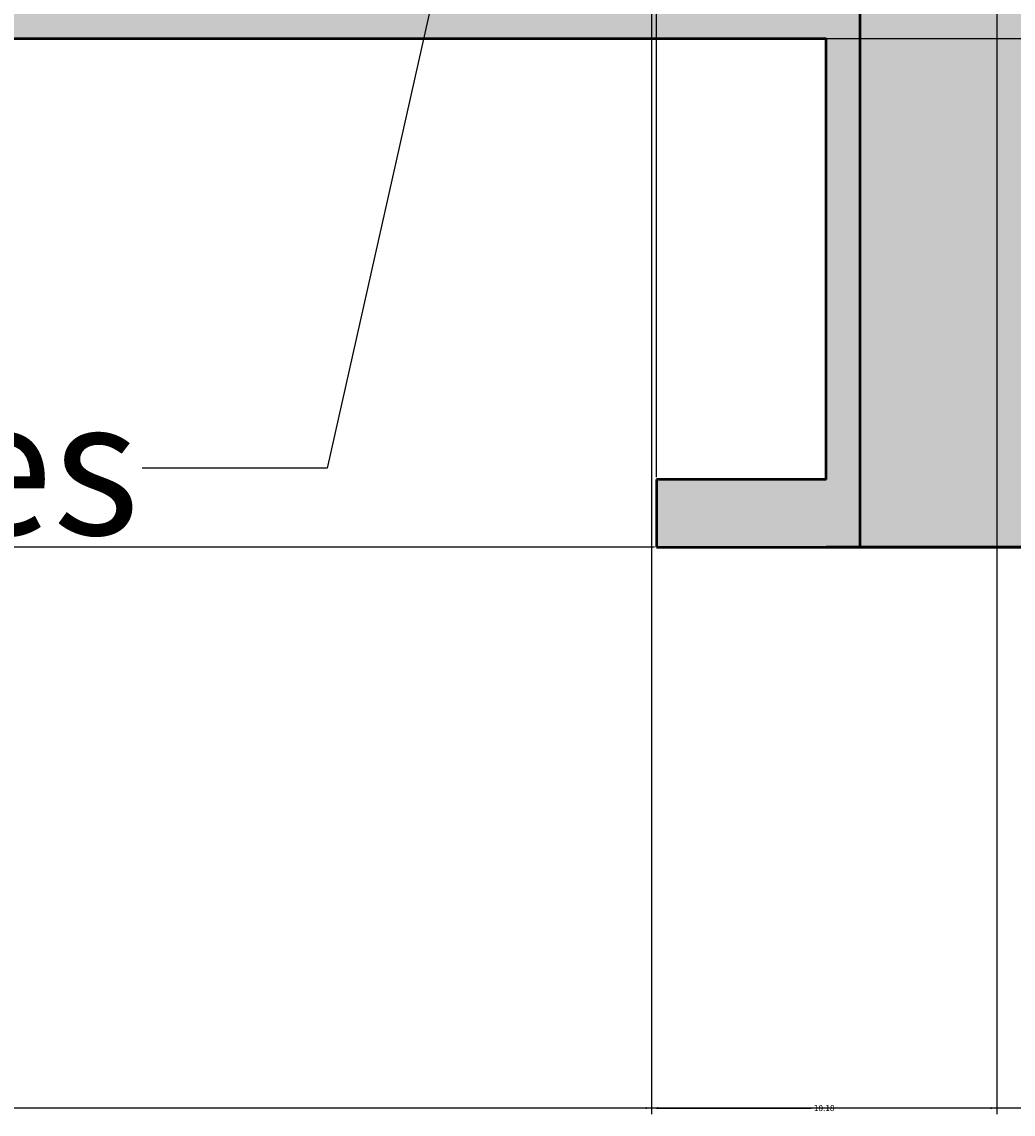
# Model space of a CAD drawing. Units: inches. Extents: x -12 to 334, y -10 to 186.
# Tile 47 of 77: x 198 to 227, y 14 to 46. Entities that reach past the tile are written whole.
import ezdxf
from ezdxf import colors
from ezdxf.entities.mleader import LeaderData, LeaderLine
from ezdxf.math import Vec2, Vec3

# ---------------------------------------------------------------- set-up
doc = ezdxf.new("R2010")
doc.units = ezdxf.units.IN
doc.header["$MEASUREMENT"] = 0
for name, color, linetype, lineweight in [('M-ANNO-TEXT', 3, 'Continuous', 25), ('M-DIMS', 2, 'Continuous', 18), ('M-EQPM', 7, 'Continuous', 50), ('M-EQPM-PATT', 8, 'Continuous', 18)]:
    doc.layers.add(name, color=color, linetype=linetype, lineweight=lineweight)
doc.styles.get("Standard").update_dxf_attribs({"font": 'arial.ttf'})
doc.dimstyles.get("Standard").update_dxf_attribs({"dimtxt": 0.18, "dimasz": 0.18, "dimexe": 0.18, "dimexo": 0.0625, "dimgap": 0.09, "dimtad": 0, "dimtih": 1, "dimtoh": 1, "dimdec": 4, "dimzin": 0, "dimdsep": 46, "dimtxsty": 'Standard', "dimcen": 0.09, "dimadec": 0, "dimazin": 0, "dimtfac": 1, "dimtdec": 4, "dimtofl": 0, "dimtmove": 0, "dimatfit": 3, "dimfxl": 1, "dimtolj": 1, "dimtzin": 0, "dimarcsym": 0})

# ---------------------------------------------------------------- blocks, each defined once
blk = doc.blocks.new('*D1')
at = {"layer": 'Defpoints', "color": 0, "transparency": 16777216}
for p in [(281.426, 91.899), (3.376, 80.692), (281.426, 14.304)]:
    blk.add_point(p, dxfattribs=at)
at = {"layer": 'M-DIMS', "color": 0, "lineweight": -2, "transparency": 16777216}
for p, q in [((281.426, 91.836), (281.426, 14.124)), ((3.376, 80.629), (3.376, 14.124)), ((3.556, 14.304), (141.935, 14.304)), ((281.246, 14.304), (142.867, 14.304))]:
    blk.add_line(p, q, dxfattribs=at)
at = {"layer": 'M-DIMS', "color": 0, "transparency": 16777216}
for points in [[(3.556, 14.334), (3.556, 14.274), (3.376, 14.304)], [(281.246, 14.334), (281.246, 14.274), (281.426, 14.304)]]:
    blk.add_solid(points, dxfattribs=at)
at = {"layer": 'M-DIMS', "color": 0, "transparency": 16777216, "insert": (142.401, 14.304), "char_height": 0.18, "attachment_point": 5}
blk.add_mtext('\\A1;278.05', dxfattribs=at)
blk = doc.blocks.new('*D27')
at = {"layer": 'Defpoints', "color": 0, "transparency": 16777216}
for p in [(238.576, 169.385), (216.576, 32.854), (238.576, 32.854)]:
    blk.add_point(p, dxfattribs=at)
at = {"layer": 'M-DIMS', "color": 0, "lineweight": -2, "transparency": 16777216}
for p, q in [((216.576, 32.917), (216.576, 169.565)), ((238.576, 32.917), (238.576, 169.565)), ((216.756, 169.385), (227.357, 169.385)), ((238.396, 169.385), (227.796, 169.385))]:
    blk.add_line(p, q, dxfattribs=at)
at = {"layer": 'M-DIMS', "color": 0, "transparency": 16777216}
for points in [[(216.756, 169.415), (216.756, 169.355), (216.576, 169.385)], [(238.396, 169.415), (238.396, 169.355), (238.576, 169.385)]]:
    blk.add_solid(points, dxfattribs=at)
at = {"layer": 'M-DIMS', "color": 0, "transparency": 16777216, "insert": (227.576, 169.385), "char_height": 0.18, "attachment_point": 5}
blk.add_mtext('\\A1;22', dxfattribs=at)
blk = doc.blocks.new('*D28')
at = {"layer": 'Defpoints', "color": 0, "transparency": 16777216}
for p in [(232.576, 169.385), (222.576, 30.854), (232.576, 30.854)]:
    blk.add_point(p, dxfattribs=at)
at = {"layer": 'M-DIMS', "color": 0, "lineweight": -2, "transparency": 16777216}
for p, q in [((222.576, 30.917), (222.576, 169.565)), ((232.576, 30.917), (232.576, 169.565)), ((222.756, 169.385), (227.366, 169.385)), ((232.396, 169.385), (227.786, 169.385))]:
    blk.add_line(p, q, dxfattribs=at)
at = {"layer": 'M-DIMS', "color": 0, "transparency": 16777216}
for points in [[(222.756, 169.415), (222.756, 169.355), (222.576, 169.385)], [(232.396, 169.415), (232.396, 169.355), (232.576, 169.385)]]:
    blk.add_solid(points, dxfattribs=at)
at = {"layer": 'M-DIMS', "color": 0, "transparency": 16777216, "insert": (227.576, 169.385), "char_height": 0.18, "attachment_point": 5}
blk.add_mtext('\\A1;10', dxfattribs=at)
blk = doc.blocks.new('*D29')
at = {"layer": 'Defpoints', "color": 0, "transparency": 16777216}
for p in [(-11.174, 45.854), (221.576, 45.854), (216.576, 30.854)]:
    blk.add_point(p, dxfattribs=at)
at = {"layer": 'M-DIMS', "color": 0, "lineweight": -2, "transparency": 16777216}
for p, q in [((221.514, 45.854), (-11.354, 45.854)), ((-11.174, 45.674), (-11.174, 38.536)), ((-11.174, 31.034), (-11.174, 38.172)), ((216.514, 30.854), (-11.354, 30.854))]:
    blk.add_line(p, q, dxfattribs=at)
at = {"layer": 'M-DIMS', "color": 0, "transparency": 16777216}
for points in [[(-11.204, 45.674), (-11.144, 45.674), (-11.174, 45.854)], [(-11.204, 31.034), (-11.144, 31.034), (-11.174, 30.854)]]:
    blk.add_solid(points, dxfattribs=at)
at = {"layer": 'M-DIMS', "color": 0, "transparency": 16777216, "insert": (-11.174, 38.354), "char_height": 0.18, "attachment_point": 5}
blk.add_mtext('\\A1;15', dxfattribs=at)
blk = doc.blocks.new('*D32')
at = {"layer": 'Defpoints', "color": 0, "transparency": 16777216}
for p in [(170.908, 61.105), (216.428, 61.105), (216.428, 14.304)]:
    blk.add_point(p, dxfattribs=at)
at = {"layer": 'M-DIMS', "color": 0, "lineweight": -2, "transparency": 16777216}
for p, q in [((170.908, 61.042), (170.908, 14.124)), ((216.428, 61.042), (216.428, 14.124)), ((171.088, 14.304), (193.271, 14.304)), ((216.248, 14.304), (194.064, 14.304))]:
    blk.add_line(p, q, dxfattribs=at)
at = {"layer": 'M-DIMS', "color": 0, "transparency": 16777216}
for points in [[(171.088, 14.334), (171.088, 14.274), (170.908, 14.304)], [(216.248, 14.334), (216.248, 14.274), (216.428, 14.304)]]:
    blk.add_solid(points, dxfattribs=at)
at = {"layer": 'M-DIMS', "color": 0, "transparency": 16777216, "insert": (193.668, 14.304), "char_height": 0.18, "attachment_point": 5}
blk.add_mtext('\\A1;45.52', dxfattribs=at)
blk = doc.blocks.new('*D33')
at = {"layer": 'Defpoints', "color": 0, "transparency": 16777216}
for p in [(226.608, 79.754), (216.428, 61.105), (226.608, 14.304)]:
    blk.add_point(p, dxfattribs=at)
at = {"layer": 'M-DIMS', "color": 0, "lineweight": -2, "transparency": 16777216}
for p, q in [((226.608, 79.692), (226.608, 14.124)), ((216.428, 61.042), (216.428, 14.124)), ((216.608, 14.304), (221.133, 14.304)), ((226.428, 14.304), (221.903, 14.304))]:
    blk.add_line(p, q, dxfattribs=at)
at = {"layer": 'M-DIMS', "color": 0, "transparency": 16777216}
for points in [[(216.608, 14.334), (216.608, 14.274), (216.428, 14.304)], [(226.428, 14.334), (226.428, 14.274), (226.608, 14.304)]]:
    blk.add_solid(points, dxfattribs=at)
at = {"layer": 'M-DIMS', "color": 0, "transparency": 16777216, "insert": (221.518, 14.304), "char_height": 0.18, "attachment_point": 5}
blk.add_mtext('\\A1;10.18', dxfattribs=at)
blk = doc.blocks.new('*D39')
at = {"layer": 'Defpoints', "color": 0, "transparency": 16777216}
for p in [(279.726, 80.692), (-11.174, 45.854), (269.381, 45.854)]:
    blk.add_point(p, dxfattribs=at)
at = {"layer": 'M-DIMS', "color": 0, "lineweight": -2, "transparency": 16777216}
for p, q in [((279.664, 80.692), (-11.354, 80.692)), ((-11.174, 80.512), (-11.174, 63.455)), ((-11.174, 46.034), (-11.174, 63.091)), ((269.318, 45.854), (-11.354, 45.854))]:
    blk.add_line(p, q, dxfattribs=at)
at = {"layer": 'M-DIMS', "color": 0, "transparency": 16777216}
for points in [[(-11.204, 80.512), (-11.144, 80.512), (-11.174, 80.692)], [(-11.204, 46.034), (-11.144, 46.034), (-11.174, 45.854)]]:
    blk.add_solid(points, dxfattribs=at)
at = {"layer": 'M-DIMS', "color": 0, "transparency": 16777216, "insert": (-11.174, 63.273), "char_height": 0.18, "attachment_point": 5}
blk.add_mtext('\\A1;34.84', dxfattribs=at)

msp = doc.modelspace()

# ---------------------------------------------------------------- hatches: boundary and pattern name
at = {"layer": 'M-EQPM-PATT'}
h = msp.add_hatch(color=256, dxfattribs=at)
h.set_gradient(color1=(99, 100, 102), color2=(99, 100, 102), tint=1)
h.paths.add_polyline_path([(4.3766, 80.754, -0.4132606), (23.5807, 99.8958), (37.1002, 99.8958), (37.1002, 127.7078), (32.1002, 127.7078), (32.1002, 125.2078), (36.1002, 125.2078), (36.1002, 100.8958), (23.5807, 100.8958, 1), (23.5807, 60.4872), (36.1002, 60.4872), (36.1002, 36.1752), (32.1002, 36.1752), (32.1002, 33.6752), (37.1002, 33.6752), (37.1002, 61.4872), (23.5807, 61.4872, -0.384914), (4.4744, 78.754), (72.9244, 78.754), (72.9244, 69.6117), (75.9244, 69.6117), (75.9244, 89.8963), (72.9244, 89.8963), (72.9244, 80.754)])
h.paths.add_polyline_path([(54.1002, 125.2078), (58.1002, 125.2078), (58.1002, 127.7078), (53.1002, 127.7078), (53.1002, 99.8958), (64.5, 99.8958), (64.5, 109.0583), (63.5, 109.0583), (63.5, 100.8958), (54.1002, 100.8958)], flags=17)
h.paths.add_polyline_path([(53.1002, 33.6752), (58.1002, 33.6752), (58.1002, 36.1752), (54.1002, 36.1752), (54.1002, 60.4872), (64.2068, 60.4872), (64.2068, 49.4497), (87.8879, 49.4497), (87.8879, 55.3205), (104.8919, 55.3205), (104.8919, 30.8541), (99.8919, 30.8541), (99.8919, 28.8541), (105.8919, 28.8541), (105.8919, 56.3205), (87.8879, 56.3205), (87.8879, 63.6117), (86.8879, 63.6117), (86.8879, 50.4497), (65.0061, 50.4497), (65.0061, 63.6117), (64.5, 63.6117), (64.5, 61.4872), (53.1002, 61.4872)])
h.paths.add_polyline_path([(121.8919, 28.8541), (121.8919, 30.8541), (116.8919, 30.8541), (116.8919, 45.8541), (209.6965, 45.8541), (209.9204, 46.8541), (115.8919, 46.8541), (115.8919, 28.8541)])
h.paths.add_polyline_path([(221.5761, 32.8541), (216.5761, 32.8541), (216.5761, 30.8541), (222.5761, 30.8541), (222.5761, 46.8541), (209.9204, 46.8541), (209.6965, 45.8541), (221.5761, 45.8541)])
h.paths.add_polyline_path([(233.5761, 45.8541), (249.8485, 45.8541), (249.3759, 46.8541), (232.5761, 46.8541), (232.5761, 30.8541), (238.5761, 30.8541), (238.5761, 32.8541), (233.5761, 32.8541)])
h = msp.add_hatch(color=256, dxfattribs=at)
h.set_gradient(color1=(94, 103, 175), color2=(94, 103, 175), tint=1)
h.paths.add_polyline_path([(129.093, 89.8963), (86.8879, 89.8963), (86.8879, 69.6117), (129.093, 69.6117)], flags=17)
h.paths.add_polyline_path([(170.9079, 89.8963), (130.8573, 89.8963), (130.8573, 69.6117), (170.9079, 69.6117)], flags=17)
h.paths.add_polyline_path([(216.4278, 89.8963), (172.6722, 89.8963), (172.6722, 69.6117), (216.4278, 69.6117)], flags=17)
h.paths.add_polyline_path([(245.9354, 82.6969), (247.9354, 82.6969), (247.9354, 46.8541), (268.3808, 46.8541, 0.0998398), (279.7263, 80.6915), (251.9801, 80.6915, 0.4142136), (231.7758, 100.8958), (84.7229, 100.8958), (84.7229, 109.0583), (83.7229, 109.0583), (83.7229, 95.8963), (129.093, 95.8963), (129.093, 98.1081), (130.8573, 98.1081), (130.8573, 95.8963), (170.9079, 95.8963), (170.9079, 98.1081), (172.6722, 98.1081), (172.6722, 95.8963), (216.4278, 95.8963), (216.4278, 98.1081), (218.1922, 98.1081), (218.1922, 95.8963), (226.6083, 95.8963, -1), (226.6083, 63.6117), (218.1922, 63.6117), (218.1922, 61.1045), (216.4278, 61.1045), (216.4278, 63.6117), (172.6722, 63.6117), (172.6722, 61.1045), (170.9079, 61.1045), (170.9079, 63.6117), (130.8573, 63.6117), (130.8573, 61.1045), (129.093, 61.1045), (129.093, 63.6117), (87.8879, 63.6117), (87.8879, 56.3205), (105.8919, 56.3205), (105.8919, 28.8541), (115.8919, 28.8541), (115.8919, 46.8541), (222.5761, 46.8541), (222.5761, 30.8541), (232.5761, 30.8541), (232.5761, 46.8541), (245.9354, 46.8541)])
h.paths.add_polyline_path([(86.8879, 89.8963), (75.9244, 89.8963), (75.9244, 69.6117), (86.8879, 69.6117)])
h.paths.add_polyline_path([(83.7229, 109.0583), (75.9244, 109.0583), (75.9244, 95.8963), (83.7229, 95.8963)])
h.paths.add_polyline_path([(226.6083, 89.8963), (218.1922, 89.8963), (218.1922, 69.6117), (226.6083, 69.6117, 1)], flags=17)
h = msp.add_hatch(color=256, dxfattribs=at)
h.set_gradient(color1=(0, 0, 255), color2=(0, 0, 255), tint=1)
h.paths.add_polyline_path([(84.7229, 100.8958), (84.7229, 109.0583), (83.7229, 109.0583), (83.7229, 95.8963), (129.093, 95.8963), (129.093, 98.1081), (130.8573, 98.1081), (130.8573, 95.8963), (170.9079, 95.8963), (170.9079, 98.1081), (172.6722, 98.1081), (172.6722, 95.8963), (216.4278, 95.8963), (216.4278, 98.1081), (218.1922, 98.1081), (218.1922, 95.8963), (226.6083, 95.8963, -1), (226.6083, 63.6117), (218.1922, 63.6117), (218.1922, 61.1045), (216.4278, 61.1045), (216.4278, 63.6117), (172.6722, 63.6117), (172.6722, 61.1045), (170.9079, 61.1045), (170.9079, 63.6117), (130.8573, 63.6117), (130.8573, 61.1045), (129.093, 61.1045), (129.093, 63.6117), (87.8879, 63.6117), (87.8879, 56.3205), (105.8919, 56.3205), (105.8919, 28.8541), (115.8919, 28.8541), (115.8919, 46.8541), (222.5761, 46.8541), (222.5761, 30.8541), (232.5761, 30.8541), (232.5761, 46.8541), (245.9354, 46.8541), (245.9354, 82.6969), (247.9354, 82.6969), (247.9354, 46.8541), (268.3808, 46.8541, 0.0998398), (279.7263, 80.6915), (251.9801, 80.6915, 0.4142136), (231.7758, 100.8958)])

# ---------------------------------------------------------------- linework, layer by layer
at = {"layer": 'M-EQPM'}
for p, q in [((222.5761, 30.8541), (222.5761, 46.8541)), ((221.5761, 45.8541), (116.8919, 45.8541)), ((221.5761, 32.8541), (221.5761, 45.8541)), ((221.5761, 32.8541), (216.5761, 32.8541)), ((216.5761, 32.8541), (216.5761, 30.8541)), ((216.5761, 30.8541), (238.5761, 30.8541)), ((233.5761, 30.8541), (221.5761, 30.8541))]:
    msp.add_line(p, q, dxfattribs=at)

# ---------------------------------------------------------------- dimensions: what is measured, and where the dimension line sits
at = {"layer": 'M-DIMS'}
for base, p1, p2, override, picture, middle in [((238.5761, 169.3845), (216.5761, 32.8541), (238.5761, 32.8541), {"dimdec": 0, "dimlfac": 1, "dimrnd": 0, "dimzin": 0, "dimdsep": 46, "dimlunit": 2}, '*D27', (227.5761, 169.3845)), ((232.5761, 169.3845), (222.5761, 30.8541), (232.5761, 30.8541), {"dimdec": 0, "dimlfac": 1, "dimrnd": 0, "dimzin": 0, "dimdsep": 46, "dimlunit": 2}, '*D28', (227.5761, 169.3845)), ((281.4256, 14.3041), (3.3765, 80.6915), (281.4256, 91.8988), {"dimdec": 2, "dimlfac": 1, "dimrnd": 0, "dimzin": 0, "dimdsep": 46, "dimlunit": 2}, '*D1', (142.401, 14.3041)), ((226.6083, 14.3041), (216.4278, 61.1045), (226.6083, 79.754), {"dimdec": 2, "dimlfac": 1, "dimrnd": 0, "dimzin": 0, "dimdsep": 46, "dimlunit": 2}, '*D33', (221.5181, 14.3041)), ((216.4278, 14.3041), (170.9079, 61.1045), (216.4278, 61.1045), {"dimdec": 2, "dimlfac": 1, "dimrnd": 0, "dimzin": 0, "dimdsep": 46, "dimlunit": 2}, '*D32', (193.6678, 14.3041))]:
    dim = msp.add_linear_dim(base=base, p1=p1, p2=p2, dimstyle='Standard', override=override, dxfattribs=at)
    dim.commit()
    dim.dimension.update_dxf_attribs({"geometry": picture, "text_midpoint": middle})
for p1, p2, override, picture, middle in [((279.7263, 80.6915), (269.3808, 45.8541), {"dimdec": 2, "dimlfac": 1, "dimrnd": 0, "dimzin": 0, "dimdsep": 46, "dimlunit": 2}, '*D39', (-11.1735, 63.2728)), ((216.5761, 30.8541), (221.5761, 45.8541), {"dimdec": 0, "dimlfac": 1, "dimrnd": 0, "dimzin": 0, "dimdsep": 46, "dimlunit": 2}, '*D29', (-11.1735, 38.3541))]:
    dim = msp.add_linear_dim(base=(-11.1736, 45.8541), p1=p1, p2=p2, angle=90, dimstyle='Standard', override=override, dxfattribs=at)
    dim.commit()
    dim.dimension.update_dxf_attribs({"geometry": picture, "text_midpoint": middle})

# ---------------------------------------------------------------- leaders
at = {"layer": 'M-ANNO-TEXT'}
ml = msp.add_multileader_mtext('Standard', dxfattribs=at)
ml.set_content('u-tubes', color=256)
ml.set_leader_properties()
ml.build(insert=Vec2(0, 0))
ml.multileader.update_dxf_attribs({"dogleg_length": 0.36, "arrow_head_size": 0.7})
ctx = ml.context
ctx.base_point, ctx.arrow_head_size, ctx.landing_gap_size, ctx.plane_origin = Vec3(183.1578, 33.1882), 0.7, 0.09, Vec3(168.0474, 30.6523)
ctx.text_align_type = 2
notes = []
notes.append((ctx, [(1, (1, 1, 0), (206.8598, 33.1882), (-1, 0), 5.4565, [(0, [(213.6735, 63.6117)], 0, [])])]))
ctx.mtext.insert, ctx.mtext.alignment, ctx.mtext.flow_direction = Vec3(201.3133, 35.2209), 3, 5
for ctx, leaders in notes:
    for number, flags, end, landing, length, lines in leaders:
        leader = LeaderData()
        leader.index, (leader.has_last_leader_line, leader.has_dogleg_vector, leader.attachment_direction) = number, flags
        leader.last_leader_point, leader.dogleg_vector, leader.dogleg_length = Vec3(end), Vec3(landing), length
        for number, points, colour, breaks in lines:
            line = LeaderLine()
            line.index, line.vertices, line.color, line.breaks = number, Vec3.list(points), colors.encode_raw_color(colour), breaks
            leader.lines.append(line)
        ctx.leaders.append(leader)

doc.saveas('drawing.dxf')
